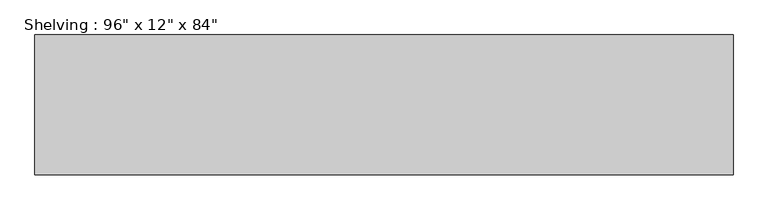
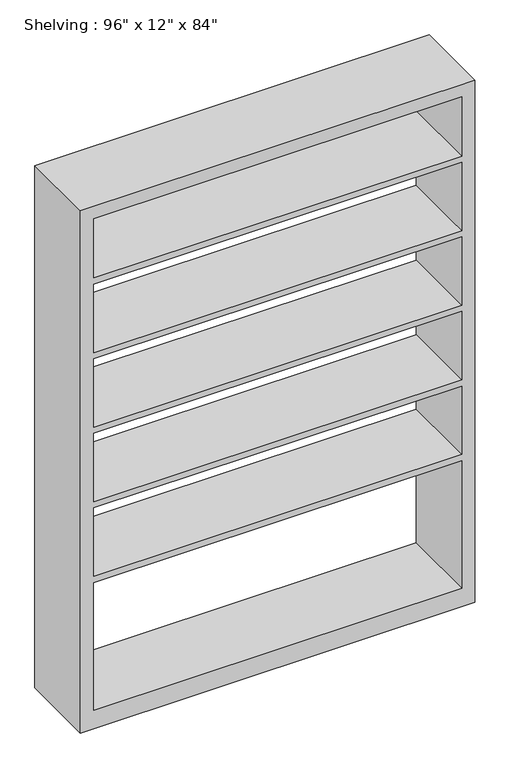
"""IFC4 building model written with IfcOpenShell, lengths in millimetres: furniture geometry."""

from ifc_helpers import new_model, si_unit, frame, origin, place, context, project, spatial, polyline, outline, extrude, source, transform, mapped, element, save


def furniture_b7bad97b(model_context):
    return source(origin(), model_context, "Body", "SweptSolid", [
        extrude(outline(polyline([(0.0, 762.0), (2133.6, 762.0), (2133.6, -762.0), (0.0, -762.0), (0.0, 762.0)]), holes=[polyline([(2082.8, 711.2), (1841.5, 711.2), (1841.5, -711.2), (2082.8, -711.2), (2082.8, 711.2)]), polyline([(76.2, 711.2), (76.2, -711.2), (596.9, -711.2), (596.9, 711.2), (76.2, 711.2)]), polyline([(1231.9, -711.2), (1511.3, -711.2), (1511.3, 711.2), (1231.9, 711.2), (1231.9, -711.2)]), polyline([(1816.1, 711.2), (1536.7, 711.2), (1536.7, -711.2), (1816.1, -711.2), (1816.1, 711.2)]), polyline([(1206.5, 711.2), (927.1, 711.2), (927.1, -711.2), (1206.5, -711.2), (1206.5, 711.2)]), polyline([(901.7, 711.2), (622.3, 711.2), (622.3, -711.2), (901.7, -711.2), (901.7, 711.2)])]), frame((0.0, -457.2, 0.0), z_axis=(0.0, 1.0, 0.0), x_axis=(0.0, 0.0, 1.0)), (0.0, 0.0, 1.0), 304.8),
    ])


if __name__ == "__main__":
    model = new_model("IFC4")
    model_context = context("Model", 3, world=origin())
    ifc_project = project(units=[si_unit("LENGTHUNIT", "METRE", prefix="MILLI")], contexts=[model_context])
    site = spatial("IfcSite", under=ifc_project)
    building = spatial("IfcBuilding", under=site)
    placement = place(None, origin())
    furniture_shape = furniture_b7bad97b(model_context)
    element("IfcFurniture", 1, ObjectType="Shelving : 96\" x 12\" x 84\"", at=placement, inside=building, context=model_context, shape_type="MappedRepresentation", body=[
        mapped(furniture_shape, transform((0.0, 0.0, 0.0), x_axis=(1.0, 0.0, 0.0), y_axis=(0.0, 1.0, 0.0), z_axis=(0.0, 0.0, 1.0))),
    ])
    save(model, "model.ifc")

# Revit data of these elements
# Type "Shelving : 96\" x 12\" x 84\""
#   Assembly Code = "E2020200"
#   Depth = 1' - 0"
#   Height = 7' - 0"
#   Width = 5' - 0"
#   Shelving Unit Material = Laminate, Ivory, Matte
#   Default Elevation = 0
# Element 1 (IfcFurniture, "Shelving : 96\" x 12\" x 84\"")
#   Materials on its faces: "Laminate, Ivory, Matte"
# Materials
#   "Laminate, Ivory, Matte": class "Plastic", colour RGB 247 247 239, transparency 0, Description = "Plastic Laminate - Ivory, Matte", Cost = 0
